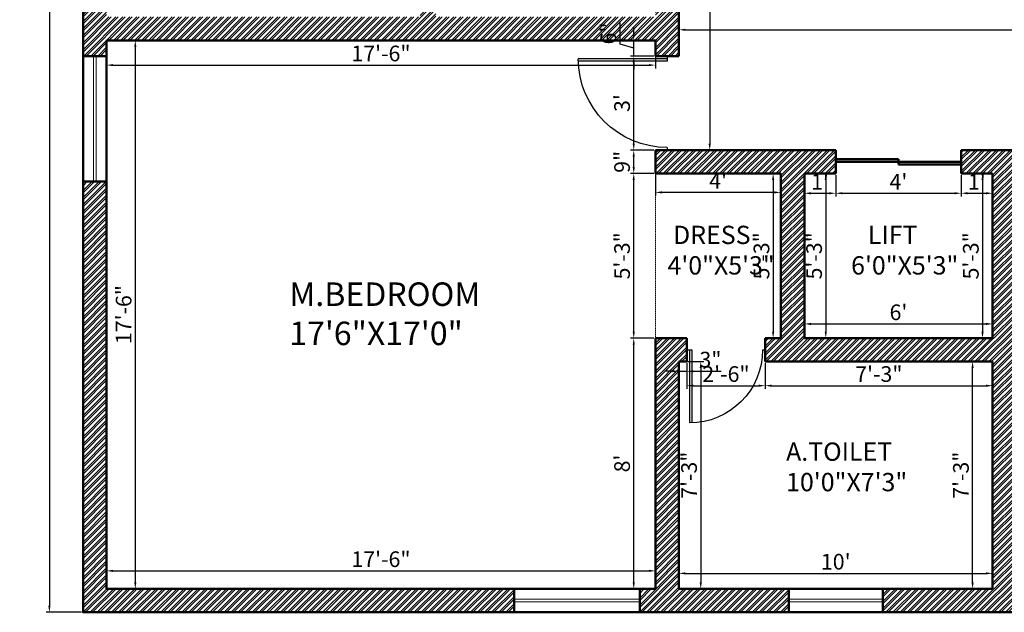
# Model space of a CAD drawing. Units: inches. Extents: x 3590 to 5167, y 65 to 1917.
# Tile 13 of 100: x 3621 to 3998, y 735 to 962. Entities that reach past the tile are written whole.
import ezdxf

# ---------------------------------------------------------------- set-up
doc = ezdxf.new("R2010")
doc.units = ezdxf.units.IN
doc.linetypes.add('DASHED', pattern=[0.75, 0.5, -0.25])
for name, color, linetype, lineweight in [('A-ANNO-DIMS', 2, 'Continuous', 18), ('A-AREA-IDEN', 7, 'Continuous', 18), ('A-DOOR', 3, 'Continuous', 25), ('A-GLAZ', 4, 'Continuous', 18), ('A-WALL', 7, 'Continuous', 50), ('A-WALL-PATT', 251, 'Continuous', 13), ('S-BEAM-OVHD', 7, 'DASHED', 18)]:
    doc.layers.add(name, color=color, linetype=linetype, lineweight=lineweight)
doc.styles.get("Standard").update_dxf_attribs({"font": 'arial.ttf'})
doc.dimstyles.new('ISO-25', dxfattribs={"dimtxt": 9, "dimasz": 2.5, "dimexe": 1.25, "dimexo": 0.625, "dimtad": 1, "dimdec": 1, "dimlunit": 3, "dimtxsty": 'Standard', "dimcen": 2.5, "dimadec": 0, "dimazin": 0, "dimtfac": 1, "dimtdec": 1, "dimtmove": 0, "dimatfit": 3, "dimfxl": 1, "dimarcsym": 0})

# ---------------------------------------------------------------- blocks, each defined once
blk = doc.blocks.new('*D10')
at = {"layer": 'A-ANNO-DIMS', "color": 0, "lineweight": -2, "transparency": 16777216}
for p, q in [((3644.89, 1215.35), (3631.39, 1215.35)), ((3632.64, 1212.85), (3632.64, 737.85)), ((3644.89, 735.35), (3631.39, 735.35))]:
    blk.add_line(p, q, dxfattribs=at)
at = {"layer": 'A-ANNO-DIMS', "color": 0, "transparency": 16777216}
for points in [[(3632.22, 1212.85), (3633.06, 1212.85), (3632.64, 1215.35)], [(3632.22, 737.85), (3633.06, 737.85), (3632.64, 735.35)]]:
    blk.add_solid(points, dxfattribs=at)
at = {"layer": 'Defpoints', "color": 0, "transparency": 16777216}
for p in [(3645.51, 1215.35), (3632.64, 735.35), (3645.51, 735.35)]:
    blk.add_point(p, dxfattribs=at)
at = {"layer": 'A-ANNO-DIMS', "color": 0, "transparency": 16777216, "insert": (3627.42, 975.35), "char_height": 9, "attachment_point": 5, "rotation": 90}
blk.add_mtext("40'", dxfattribs=at)
blk = doc.blocks.new('D2')
for p, q in [((1, 0), (1, 28)), ((2, 0), (2, 27.98)), ((0, 0), (2, 0)), ((29, 0), (30, 0))]:
    blk.add_line(p, q)
at = {"ltscale": 0.5}
blk.add_arc((1, 0), 28, 0, 90, dxfattribs=at)
blk = doc.blocks.new('D1')
for p, q in [((1, 0), (1, 34)), ((2, 0), (2, 33.99)), ((0, 0), (2, 0)), ((35, 0), (36, 0))]:
    blk.add_line(p, q)
at = {"ltscale": 0.5}
blk.add_arc((1, 0), 34, 0, 90, dxfattribs=at)
blk = doc.blocks.new('*D35')
at = {"layer": 'A-ANNO-DIMS', "color": 0, "lineweight": -2, "transparency": 16777216}
for p, q in [((3654.51, 953.72), (3654.51, 943.63)), ((3864.51, 953.72), (3864.51, 943.63)), ((3657.01, 944.88), (3862.01, 944.88))]:
    blk.add_line(p, q, dxfattribs=at)
at = {"layer": 'A-ANNO-DIMS', "color": 0, "transparency": 16777216}
for points in [[(3657.01, 945.3), (3657.01, 944.47), (3654.51, 944.88)], [(3862.01, 945.3), (3862.01, 944.47), (3864.51, 944.88)]]:
    blk.add_solid(points, dxfattribs=at)
at = {"layer": 'Defpoints', "color": 0, "transparency": 16777216}
for p in [(3654.51, 954.35), (3864.51, 954.35), (3864.51, 944.88)]:
    blk.add_point(p, dxfattribs=at)
at = {"layer": 'A-ANNO-DIMS', "color": 0, "transparency": 16777216, "insert": (3759.51, 948.57), "char_height": 6, "attachment_point": 5}
blk.add_mtext('17\'-6"', dxfattribs=at)
blk = doc.blocks.new('*D36')
at = {"layer": 'A-ANNO-DIMS', "color": 0, "lineweight": -2, "transparency": 16777216}
for p, q in [((3655.14, 954.35), (3666.77, 954.35)), ((3665.52, 951.85), (3665.52, 746.85)), ((3655.14, 744.35), (3666.77, 744.35))]:
    blk.add_line(p, q, dxfattribs=at)
at = {"layer": 'A-ANNO-DIMS', "color": 0, "transparency": 16777216}
for points in [[(3665.1, 951.85), (3665.94, 951.85), (3665.52, 954.35)], [(3665.1, 746.85), (3665.94, 746.85), (3665.52, 744.35)]]:
    blk.add_solid(points, dxfattribs=at)
at = {"layer": 'Defpoints', "color": 0, "transparency": 16777216}
for p in [(3654.51, 954.35), (3654.51, 744.35), (3665.52, 744.35)]:
    blk.add_point(p, dxfattribs=at)
at = {"layer": 'A-ANNO-DIMS', "color": 0, "transparency": 16777216, "insert": (3661.83, 849.35), "char_height": 6, "attachment_point": 5, "rotation": 90}
blk.add_mtext('17\'-6"', dxfattribs=at)
blk = doc.blocks.new('*D37')
at = {"layer": 'A-ANNO-DIMS', "color": 0, "lineweight": -2, "transparency": 16777216}
for p, q in [((3654.51, 744.97), (3654.51, 752.47)), ((3657.01, 751.22), (3862.01, 751.22)), ((3864.51, 744.97), (3864.51, 752.47))]:
    blk.add_line(p, q, dxfattribs=at)
at = {"layer": 'A-ANNO-DIMS', "color": 0, "transparency": 16777216}
for points in [[(3657.01, 751.64), (3657.01, 750.81), (3654.51, 751.22)], [(3862.01, 751.64), (3862.01, 750.81), (3864.51, 751.22)]]:
    blk.add_solid(points, dxfattribs=at)
at = {"layer": 'Defpoints', "color": 0, "transparency": 16777216}
for p in [(3864.51, 751.22), (3654.51, 744.35), (3864.51, 744.35)]:
    blk.add_point(p, dxfattribs=at)
at = {"layer": 'A-ANNO-DIMS', "color": 0, "transparency": 16777216, "insert": (3759.51, 754.91), "char_height": 6, "attachment_point": 5}
blk.add_mtext('17\'-6"', dxfattribs=at)
blk = doc.blocks.new('*D38')
at = {"layer": 'A-ANNO-DIMS', "color": 0, "lineweight": -2, "transparency": 16777216}
for p, q in [((3863.89, 840.35), (3854.98, 840.35)), ((3856.23, 746.85), (3856.23, 837.85)), ((3863.89, 744.35), (3854.98, 744.35))]:
    blk.add_line(p, q, dxfattribs=at)
at = {"layer": 'A-ANNO-DIMS', "color": 0, "transparency": 16777216}
for points in [[(3855.81, 837.85), (3856.64, 837.85), (3856.23, 840.35)], [(3855.81, 746.85), (3856.64, 746.85), (3856.23, 744.35)]]:
    blk.add_solid(points, dxfattribs=at)
at = {"layer": 'Defpoints', "color": 0, "transparency": 16777216}
for p in [(3856.23, 840.35), (3864.51, 840.35), (3864.51, 744.35)]:
    blk.add_point(p, dxfattribs=at)
at = {"layer": 'A-ANNO-DIMS', "color": 0, "transparency": 16777216, "insert": (3852.54, 792.35), "char_height": 6, "attachment_point": 5, "rotation": 90}
blk.add_mtext("8'", dxfattribs=at)
blk = doc.blocks.new('*D39')
at = {"layer": 'A-ANNO-DIMS', "color": 0, "lineweight": -2, "transparency": 16777216}
for p, q in [((3863.89, 903.35), (3854.98, 903.35)), ((3856.23, 842.85), (3856.23, 900.85)), ((3863.89, 840.35), (3854.98, 840.35))]:
    blk.add_line(p, q, dxfattribs=at)
at = {"layer": 'A-ANNO-DIMS', "color": 0, "transparency": 16777216}
for points in [[(3855.81, 900.85), (3856.64, 900.85), (3856.23, 903.35)], [(3855.81, 842.85), (3856.64, 842.85), (3856.23, 840.35)]]:
    blk.add_solid(points, dxfattribs=at)
at = {"layer": 'Defpoints', "color": 0, "transparency": 16777216}
for p in [(3856.23, 903.35), (3864.51, 903.35), (3864.51, 840.35)]:
    blk.add_point(p, dxfattribs=at)
at = {"layer": 'A-ANNO-DIMS', "color": 0, "transparency": 16777216, "insert": (3852.54, 871.85), "char_height": 6, "attachment_point": 5, "rotation": 90}
blk.add_mtext('5\'-3"', dxfattribs=at)
blk = doc.blocks.new('*D40')
at = {"layer": 'A-ANNO-DIMS', "color": 0, "lineweight": -2, "transparency": 16777216}
for p, q in [((3863.89, 912.35), (3854.98, 912.35)), ((3856.23, 905.85), (3856.23, 909.85)), ((3863.89, 903.35), (3854.98, 903.35))]:
    blk.add_line(p, q, dxfattribs=at)
at = {"layer": 'A-ANNO-DIMS', "color": 0, "transparency": 16777216}
for points in [[(3855.81, 909.85), (3856.64, 909.85), (3856.23, 912.35)], [(3855.81, 905.85), (3856.64, 905.85), (3856.23, 903.35)]]:
    blk.add_solid(points, dxfattribs=at)
at = {"layer": 'Defpoints', "color": 0, "transparency": 16777216}
for p in [(3856.23, 912.35), (3864.51, 912.35), (3864.51, 903.35)]:
    blk.add_point(p, dxfattribs=at)
at = {"layer": 'A-ANNO-DIMS', "color": 0, "transparency": 16777216, "insert": (3852.54, 907.85), "char_height": 6, "attachment_point": 5, "rotation": 90}
blk.add_mtext('9"', dxfattribs=at)
blk = doc.blocks.new('*D41')
at = {"layer": 'A-ANNO-DIMS', "color": 0, "lineweight": -2, "transparency": 16777216}
for p, q in [((3863.89, 948.35), (3854.98, 948.35)), ((3856.23, 914.85), (3856.23, 945.85)), ((3863.89, 912.35), (3854.98, 912.35))]:
    blk.add_line(p, q, dxfattribs=at)
at = {"layer": 'A-ANNO-DIMS', "color": 0, "transparency": 16777216}
for points in [[(3855.81, 945.85), (3856.64, 945.85), (3856.23, 948.35)], [(3855.81, 914.85), (3856.64, 914.85), (3856.23, 912.35)]]:
    blk.add_solid(points, dxfattribs=at)
at = {"layer": 'Defpoints', "color": 0, "transparency": 16777216}
for p in [(3856.23, 948.35), (3864.51, 948.35), (3864.51, 912.35)]:
    blk.add_point(p, dxfattribs=at)
at = {"layer": 'A-ANNO-DIMS', "color": 0, "transparency": 16777216, "insert": (3852.54, 930.35), "char_height": 6, "attachment_point": 5, "rotation": 90}
blk.add_mtext("3'", dxfattribs=at)
blk = doc.blocks.new('*D42')
at = {"layer": 'A-ANNO-DIMS', "color": 0, "lineweight": -2, "transparency": 16777216}
for p, q in [((3850.98, 952.92), (3850.98, 961.1)), ((3856.23, 956.85), (3856.23, 959.35)), ((3863.89, 954.35), (3854.98, 954.35)), ((3856.23, 948.35), (3856.23, 954.35)), ((3856.23, 948.35), (3856.23, 954.35)), ((3856.23, 951.35), (3850.98, 952.92)), ((3863.89, 948.35), (3854.98, 948.35)), ((3856.23, 945.85), (3856.23, 943.35))]:
    blk.add_line(p, q, dxfattribs=at)
at = {"layer": 'A-ANNO-DIMS', "color": 0, "transparency": 16777216}
for points in [[(3855.81, 956.85), (3856.64, 956.85), (3856.23, 954.35)], [(3855.81, 945.85), (3856.64, 945.85), (3856.23, 948.35)]]:
    blk.add_solid(points, dxfattribs=at)
at = {"layer": 'Defpoints', "color": 0, "transparency": 16777216}
for p in [(3856.23, 954.35), (3864.51, 954.35), (3864.51, 948.35)]:
    blk.add_point(p, dxfattribs=at)
at = {"layer": 'A-ANNO-DIMS', "color": 0, "transparency": 16777216, "insert": (3847.29, 957.01), "char_height": 6, "attachment_point": 5, "rotation": 90}
blk.add_mtext('6"', dxfattribs=at)
blk = doc.blocks.new('*D43')
at = {"layer": 'A-ANNO-DIMS', "color": 0, "lineweight": -2, "transparency": 16777216}
for p, q in [((3864.51, 902.72), (3864.51, 894.9)), ((3912.51, 902.72), (3912.51, 894.9)), ((3910.01, 896.15), (3867.01, 896.15))]:
    blk.add_line(p, q, dxfattribs=at)
at = {"layer": 'A-ANNO-DIMS', "color": 0, "transparency": 16777216}
for points in [[(3867.01, 896.56), (3867.01, 895.73), (3864.51, 896.15)], [(3910.01, 896.56), (3910.01, 895.73), (3912.51, 896.15)]]:
    blk.add_solid(points, dxfattribs=at)
at = {"layer": 'Defpoints', "color": 0, "transparency": 16777216}
for p in [(3864.51, 903.35), (3912.51, 903.35), (3864.51, 896.15)]:
    blk.add_point(p, dxfattribs=at)
at = {"layer": 'A-ANNO-DIMS', "color": 0, "transparency": 16777216, "insert": (3888.51, 899.77), "char_height": 6, "attachment_point": 5}
blk.add_mtext("4'", dxfattribs=at)
blk = doc.blocks.new('*D44')
at = {"layer": 'A-ANNO-DIMS', "color": 0, "lineweight": -2, "transparency": 16777216}
for p, q in [((3911.89, 903.35), (3908.31, 903.35)), ((3909.56, 900.85), (3909.56, 842.85)), ((3911.89, 840.35), (3908.31, 840.35))]:
    blk.add_line(p, q, dxfattribs=at)
at = {"layer": 'A-ANNO-DIMS', "color": 0, "transparency": 16777216}
for points in [[(3909.14, 900.85), (3909.98, 900.85), (3909.56, 903.35)], [(3909.14, 842.85), (3909.98, 842.85), (3909.56, 840.35)]]:
    blk.add_solid(points, dxfattribs=at)
at = {"layer": 'Defpoints', "color": 0, "transparency": 16777216}
for p in [(3912.51, 903.35), (3909.56, 840.35), (3912.51, 840.35)]:
    blk.add_point(p, dxfattribs=at)
at = {"layer": 'A-ANNO-DIMS', "color": 0, "transparency": 16777216, "insert": (3905.87, 871.85), "char_height": 6, "attachment_point": 5, "rotation": 90}
blk.add_mtext('5\'-3"', dxfattribs=at)
blk = doc.blocks.new('*D45')
at = {"layer": 'A-ANNO-DIMS', "color": 0, "lineweight": -2, "transparency": 16777216}
for p, q in [((3873.51, 830.72), (3873.51, 826.4)), ((3876.51, 830.72), (3876.51, 826.4)), ((3871.01, 827.65), (3868.51, 827.65)), ((3873.51, 827.65), (3876.51, 827.65)), ((3879.01, 827.65), (3889.65, 827.65))]:
    blk.add_line(p, q, dxfattribs=at)
at = {"layer": 'A-ANNO-DIMS', "color": 0, "transparency": 16777216}
for points in [[(3871.01, 828.07), (3871.01, 827.24), (3873.51, 827.65)], [(3879.01, 828.07), (3879.01, 827.24), (3876.51, 827.65)]]:
    blk.add_solid(points, dxfattribs=at)
at = {"layer": 'Defpoints', "color": 0, "transparency": 16777216}
for p in [(3873.51, 831.35), (3876.51, 831.35), (3876.51, 827.65)]:
    blk.add_point(p, dxfattribs=at)
at = {"layer": 'A-ANNO-DIMS', "color": 0, "transparency": 16777216, "insert": (3885.58, 831.34), "char_height": 6, "attachment_point": 5}
blk.add_mtext('3"', dxfattribs=at)
blk = doc.blocks.new('*D46')
at = {"layer": 'A-ANNO-DIMS', "color": 0, "lineweight": -2, "transparency": 16777216}
for p, q in [((3876.51, 830.72), (3876.51, 820.87)), ((3906.51, 830.72), (3906.51, 820.87)), ((3879.01, 822.12), (3904.01, 822.12))]:
    blk.add_line(p, q, dxfattribs=at)
at = {"layer": 'A-ANNO-DIMS', "color": 0, "transparency": 16777216}
for points in [[(3879.01, 822.54), (3879.01, 821.7), (3876.51, 822.12)], [(3904.01, 822.54), (3904.01, 821.7), (3906.51, 822.12)]]:
    blk.add_solid(points, dxfattribs=at)
at = {"layer": 'Defpoints', "color": 0, "transparency": 16777216}
for p in [(3876.51, 831.35), (3906.51, 831.35), (3906.51, 822.12)]:
    blk.add_point(p, dxfattribs=at)
at = {"layer": 'A-ANNO-DIMS', "color": 0, "transparency": 16777216, "insert": (3891.51, 825.81), "char_height": 6, "attachment_point": 5}
blk.add_mtext('2\'-6"', dxfattribs=at)
blk = doc.blocks.new('*D47')
at = {"layer": 'A-ANNO-DIMS', "color": 0, "lineweight": -2, "transparency": 16777216}
for p, q in [((3906.51, 830.72), (3906.51, 820.87)), ((3993.51, 830.72), (3993.51, 820.87)), ((3909.01, 822.12), (3991.01, 822.12))]:
    blk.add_line(p, q, dxfattribs=at)
at = {"layer": 'A-ANNO-DIMS', "color": 0, "transparency": 16777216}
for points in [[(3909.01, 822.54), (3909.01, 821.7), (3906.51, 822.12)], [(3991.01, 822.54), (3991.01, 821.7), (3993.51, 822.12)]]:
    blk.add_solid(points, dxfattribs=at)
at = {"layer": 'Defpoints', "color": 0, "transparency": 16777216}
for p in [(3906.51, 831.35), (3993.51, 831.35), (3993.51, 822.12)]:
    blk.add_point(p, dxfattribs=at)
at = {"layer": 'A-ANNO-DIMS', "color": 0, "transparency": 16777216, "insert": (3950.01, 825.81), "char_height": 6, "attachment_point": 5}
blk.add_mtext('7\'-3"', dxfattribs=at)
blk = doc.blocks.new('*D48')
at = {"layer": 'A-ANNO-DIMS', "color": 0, "lineweight": -2, "transparency": 16777216}
for p, q in [((3874.14, 831.35), (3883.11, 831.35)), ((3881.86, 828.85), (3881.86, 746.85)), ((3874.14, 744.35), (3883.11, 744.35))]:
    blk.add_line(p, q, dxfattribs=at)
at = {"layer": 'A-ANNO-DIMS', "color": 0, "transparency": 16777216}
for points in [[(3881.44, 828.85), (3882.28, 828.85), (3881.86, 831.35)], [(3881.44, 746.85), (3882.28, 746.85), (3881.86, 744.35)]]:
    blk.add_solid(points, dxfattribs=at)
at = {"layer": 'Defpoints', "color": 0, "transparency": 16777216}
for p in [(3873.51, 831.35), (3873.51, 744.35), (3881.86, 744.35)]:
    blk.add_point(p, dxfattribs=at)
at = {"layer": 'A-ANNO-DIMS', "color": 0, "transparency": 16777216, "insert": (3878.17, 787.85), "char_height": 6, "attachment_point": 5, "rotation": 90}
blk.add_mtext('7\'-3"', dxfattribs=at)
blk = doc.blocks.new('*D49')
at = {"layer": 'A-ANNO-DIMS', "color": 0, "lineweight": -2, "transparency": 16777216}
for p, q in [((3873.51, 744.97), (3873.51, 751.51)), ((3876.01, 750.26), (3991.01, 750.26)), ((3993.51, 744.97), (3993.51, 751.51))]:
    blk.add_line(p, q, dxfattribs=at)
at = {"layer": 'A-ANNO-DIMS', "color": 0, "transparency": 16777216}
for points in [[(3876.01, 750.68), (3876.01, 749.84), (3873.51, 750.26)], [(3991.01, 750.68), (3991.01, 749.84), (3993.51, 750.26)]]:
    blk.add_solid(points, dxfattribs=at)
at = {"layer": 'Defpoints', "color": 0, "transparency": 16777216}
for p in [(3993.51, 750.26), (3873.51, 744.35), (3993.51, 744.35)]:
    blk.add_point(p, dxfattribs=at)
at = {"layer": 'A-ANNO-DIMS', "color": 0, "transparency": 16777216, "insert": (3933.51, 753.95), "char_height": 6, "attachment_point": 5}
blk.add_mtext("10'", dxfattribs=at)
blk = doc.blocks.new('*D50')
at = {"layer": 'A-ANNO-DIMS', "color": 0, "lineweight": -2, "transparency": 16777216}
for p, q in [((3992.89, 831.35), (3984.62, 831.35)), ((3985.87, 746.85), (3985.87, 828.85)), ((3992.89, 744.35), (3984.62, 744.35))]:
    blk.add_line(p, q, dxfattribs=at)
at = {"layer": 'A-ANNO-DIMS', "color": 0, "transparency": 16777216}
for points in [[(3985.45, 828.85), (3986.29, 828.85), (3985.87, 831.35)], [(3985.45, 746.85), (3986.29, 746.85), (3985.87, 744.35)]]:
    blk.add_solid(points, dxfattribs=at)
at = {"layer": 'Defpoints', "color": 0, "transparency": 16777216}
for p in [(3985.87, 831.35), (3993.51, 831.35), (3993.51, 744.35)]:
    blk.add_point(p, dxfattribs=at)
at = {"layer": 'A-ANNO-DIMS', "color": 0, "transparency": 16777216, "insert": (3982.18, 787.85), "char_height": 6, "attachment_point": 5, "rotation": 90}
blk.add_mtext('7\'-3"', dxfattribs=at)
blk = doc.blocks.new('*D51')
at = {"layer": 'A-ANNO-DIMS', "color": 0, "lineweight": -2, "transparency": 16777216}
for p, q in [((3921.51, 840.97), (3921.51, 847.03)), ((3924.01, 845.78), (3991.01, 845.78)), ((3993.51, 840.97), (3993.51, 847.03))]:
    blk.add_line(p, q, dxfattribs=at)
at = {"layer": 'A-ANNO-DIMS', "color": 0, "transparency": 16777216}
for points in [[(3924.01, 846.2), (3924.01, 845.37), (3921.51, 845.78)], [(3991.01, 846.2), (3991.01, 845.37), (3993.51, 845.78)]]:
    blk.add_solid(points, dxfattribs=at)
at = {"layer": 'Defpoints', "color": 0, "transparency": 16777216}
for p in [(3993.51, 845.78), (3921.51, 840.35), (3993.51, 840.35)]:
    blk.add_point(p, dxfattribs=at)
at = {"layer": 'A-ANNO-DIMS', "color": 0, "transparency": 16777216, "insert": (3957.51, 849.47), "char_height": 6, "attachment_point": 5}
blk.add_mtext("6'", dxfattribs=at)
blk = doc.blocks.new('*D52')
at = {"layer": 'A-ANNO-DIMS', "color": 0, "lineweight": -2, "transparency": 16777216}
for p, q in [((3922.14, 903.35), (3930.95, 903.35)), ((3929.7, 900.85), (3929.7, 842.85)), ((3922.14, 840.35), (3930.95, 840.35))]:
    blk.add_line(p, q, dxfattribs=at)
at = {"layer": 'A-ANNO-DIMS', "color": 0, "transparency": 16777216}
for points in [[(3929.29, 900.85), (3930.12, 900.85), (3929.7, 903.35)], [(3929.29, 842.85), (3930.12, 842.85), (3929.7, 840.35)]]:
    blk.add_solid(points, dxfattribs=at)
at = {"layer": 'Defpoints', "color": 0, "transparency": 16777216}
for p in [(3921.51, 903.35), (3921.51, 840.35), (3929.7, 840.35)]:
    blk.add_point(p, dxfattribs=at)
at = {"layer": 'A-ANNO-DIMS', "color": 0, "transparency": 16777216, "insert": (3926.01, 871.85), "char_height": 6, "attachment_point": 5, "rotation": 90}
blk.add_mtext('5\'-3"', dxfattribs=at)
blk = doc.blocks.new('*D53')
at = {"layer": 'A-ANNO-DIMS', "color": 0, "lineweight": -2, "transparency": 16777216}
for p, q in [((3992.89, 903.35), (3988.42, 903.35)), ((3989.67, 900.85), (3989.67, 842.85)), ((3992.89, 840.35), (3988.42, 840.35))]:
    blk.add_line(p, q, dxfattribs=at)
at = {"layer": 'A-ANNO-DIMS', "color": 0, "transparency": 16777216}
for points in [[(3989.25, 900.85), (3990.09, 900.85), (3989.67, 903.35)], [(3989.25, 842.85), (3990.09, 842.85), (3989.67, 840.35)]]:
    blk.add_solid(points, dxfattribs=at)
at = {"layer": 'Defpoints', "color": 0, "transparency": 16777216}
for p in [(3993.51, 903.35), (3989.67, 840.35), (3993.51, 840.35)]:
    blk.add_point(p, dxfattribs=at)
at = {"layer": 'A-ANNO-DIMS', "color": 0, "transparency": 16777216, "insert": (3985.98, 871.85), "char_height": 6, "attachment_point": 5, "rotation": 90}
blk.add_mtext('5\'-3"', dxfattribs=at)
blk = doc.blocks.new('*D54')
at = {"layer": 'A-ANNO-DIMS', "color": 0, "lineweight": -2, "transparency": 16777216}
for p, q in [((3921.51, 902.72), (3921.51, 894.56)), ((3933.51, 902.72), (3933.51, 894.56)), ((3924.01, 895.81), (3931.01, 895.81))]:
    blk.add_line(p, q, dxfattribs=at)
at = {"layer": 'A-ANNO-DIMS', "color": 0, "transparency": 16777216}
for points in [[(3924.01, 896.23), (3924.01, 895.4), (3921.51, 895.81)], [(3931.01, 896.23), (3931.01, 895.4), (3933.51, 895.81)]]:
    blk.add_solid(points, dxfattribs=at)
at = {"layer": 'Defpoints', "color": 0, "transparency": 16777216}
for p in [(3921.51, 903.35), (3933.51, 903.35), (3933.51, 895.81)]:
    blk.add_point(p, dxfattribs=at)
at = {"layer": 'A-ANNO-DIMS', "color": 0, "transparency": 16777216, "insert": (3927.51, 899.45), "char_height": 6, "attachment_point": 5}
blk.add_mtext("1'", dxfattribs=at)
blk = doc.blocks.new('*D55')
at = {"layer": 'A-ANNO-DIMS', "color": 0, "lineweight": -2, "transparency": 16777216}
for p, q in [((3933.51, 902.72), (3933.51, 894.56)), ((3981.51, 902.72), (3981.51, 894.56)), ((3936.01, 895.81), (3979.01, 895.81))]:
    blk.add_line(p, q, dxfattribs=at)
at = {"layer": 'A-ANNO-DIMS', "color": 0, "transparency": 16777216}
for points in [[(3936.01, 896.23), (3936.01, 895.4), (3933.51, 895.81)], [(3979.01, 896.23), (3979.01, 895.4), (3981.51, 895.81)]]:
    blk.add_solid(points, dxfattribs=at)
at = {"layer": 'Defpoints', "color": 0, "transparency": 16777216}
for p in [(3933.51, 903.35), (3981.51, 903.35), (3981.51, 895.81)]:
    blk.add_point(p, dxfattribs=at)
at = {"layer": 'A-ANNO-DIMS', "color": 0, "transparency": 16777216, "insert": (3957.51, 899.44), "char_height": 6, "attachment_point": 5}
blk.add_mtext("4'", dxfattribs=at)
blk = doc.blocks.new('*D56')
at = {"layer": 'A-ANNO-DIMS', "color": 0, "lineweight": -2, "transparency": 16777216}
for p, q in [((3981.51, 902.72), (3981.51, 894.56)), ((3993.51, 902.72), (3993.51, 894.56)), ((3984.01, 895.81), (3991.01, 895.81))]:
    blk.add_line(p, q, dxfattribs=at)
at = {"layer": 'A-ANNO-DIMS', "color": 0, "transparency": 16777216}
for points in [[(3984.01, 896.23), (3984.01, 895.4), (3981.51, 895.81)], [(3991.01, 896.23), (3991.01, 895.4), (3993.51, 895.81)]]:
    blk.add_solid(points, dxfattribs=at)
at = {"layer": 'Defpoints', "color": 0, "transparency": 16777216}
for p in [(3981.51, 903.35), (3993.51, 903.35), (3993.51, 895.81)]:
    blk.add_point(p, dxfattribs=at)
at = {"layer": 'A-ANNO-DIMS', "color": 0, "transparency": 16777216, "insert": (3987.51, 899.45), "char_height": 6, "attachment_point": 5}
blk.add_mtext("1'", dxfattribs=at)
blk = doc.blocks.new('*D73')
at = {"layer": 'A-ANNO-DIMS', "color": 0, "lineweight": -2, "transparency": 16777216}
for p, q in [((3874.14, 1206.35), (3886.54, 1206.35)), ((3885.29, 1203.85), (3885.29, 914.85)), ((3874.14, 912.35), (3886.54, 912.35))]:
    blk.add_line(p, q, dxfattribs=at)
at = {"layer": 'A-ANNO-DIMS', "color": 0, "transparency": 16777216}
for points in [[(3884.87, 1203.85), (3885.7, 1203.85), (3885.29, 1206.35)], [(3884.87, 914.85), (3885.7, 914.85), (3885.29, 912.35)]]:
    blk.add_solid(points, dxfattribs=at)
at = {"layer": 'Defpoints', "color": 0, "transparency": 16777216}
for p in [(3873.51, 1206.35), (3873.51, 912.35), (3885.29, 912.35)]:
    blk.add_point(p, dxfattribs=at)
at = {"layer": 'A-ANNO-DIMS', "color": 0, "transparency": 16777216, "insert": (3881.6, 1059.35), "char_height": 6, "attachment_point": 5, "rotation": 90}
blk.add_mtext('24\'-6"', dxfattribs=at)
blk = doc.blocks.new('*D74')
at = {"layer": 'A-ANNO-DIMS', "color": 0, "lineweight": -2, "transparency": 16777216}
for p, q in [((3873.51, 948.97), (3873.51, 959.67)), ((3876.01, 958.42), (4147.01, 958.42)), ((4149.51, 945.97), (4149.51, 959.67))]:
    blk.add_line(p, q, dxfattribs=at)
at = {"layer": 'A-ANNO-DIMS', "color": 0, "transparency": 16777216}
for points in [[(3876.01, 958.83), (3876.01, 958), (3873.51, 958.42)], [(4147.01, 958.83), (4147.01, 958), (4149.51, 958.42)]]:
    blk.add_solid(points, dxfattribs=at)
at = {"layer": 'Defpoints', "color": 0, "transparency": 16777216}
for p in [(4149.51, 958.42), (3873.51, 948.35), (4149.51, 945.35)]:
    blk.add_point(p, dxfattribs=at)
at = {"layer": 'A-ANNO-DIMS', "color": 0, "transparency": 16777216, "insert": (4011.51, 962.11), "char_height": 6, "attachment_point": 5}
blk.add_mtext("23'", dxfattribs=at)

msp = doc.modelspace()

# ---------------------------------------------------------------- hatches: boundary and pattern name
at = {"layer": 'A-WALL-PATT', "transparency": 33554687}
h = msp.add_hatch(dxfattribs=at)
h.set_pattern_fill('ANSI32', color=256, scale=0.2)
h.set_pattern_definition([(45, (0, -590.6538), (-1.3470384, 1.3470384), []), (45, (0.898, -590.6538), (-1.3470384, 1.3470384), [])])
h.paths.add_polyline_path([(3768.51, 1215.35), (3645.51, 1215.35), (3645.51, 1194.35), (3654.51, 1194.35), (3654.51, 1206.35), (3671.16, 1206.35), (3768.51, 1206.35)])
h.paths.add_polyline_path([(3909.51, 1215.35), (3816.51, 1215.35), (3816.51, 1206.35), (3864.51, 1206.35), (3864.51, 1200.35), (3873.51, 1200.35), (3873.51, 1206.35), (3909.51, 1206.35)])
h.paths.add_polyline_path([(4053.51, 1215.35), (3969.51, 1215.35), (3969.51, 1206.35), (4053.51, 1206.35)])
h.paths.add_polyline_path([(4215.51, 1215.35), (4113.51, 1215.35), (4113.51, 1206.35), (4206.51, 1206.35), (4206.51, 1200.35), (4215.51, 1200.35)])
h.paths.add_polyline_path([(3654.51, 1146.35), (3645.51, 1146.35), (3645.51, 1029.35), (3654.51, 1029.35), (3654.51, 1059.35), (3741.51, 1059.35), (3741.51, 1065.35), (3654.51, 1065.35)], flags=17)
h.paths.add_polyline_path([(3873.51, 1164.35), (3864.51, 1164.35), (3864.51, 1065.35), (3771.51, 1065.35), (3771.51, 1059.35), (3774.51, 1059.35), (3774.51, 963.35), (3654.51, 963.35), (3654.51, 993.35), (3645.51, 993.35), (3645.51, 948.35), (3654.51, 948.35), (3654.51, 954.35), (3864.51, 954.35), (3864.51, 948.35), (3873.51, 948.35), (3873.51, 993.35), (3864.51, 993.35), (3864.51, 963.35), (3780.51, 963.35), (3780.51, 1059.35), (3864.51, 1059.35), (3864.51, 1029.35), (3873.51, 1029.35)])
h.paths.add_polyline_path([(3654.51, 900.35), (3645.51, 900.35), (3645.51, 735.35), (3810.51, 735.35), (3810.51, 744.35), (3809.96, 744.35), (3654.51, 744.35)])
h.paths.add_polyline_path([(3915.51, 744.35), (3873.51, 744.35), (3873.51, 762.21), (3873.51, 831.35), (3876.51, 831.35), (3876.51, 840.35), (3864.51, 840.35), (3864.51, 744.35), (3858.51, 744.35), (3858.51, 735.35), (3915.51, 735.35)])
h.paths.add_polyline_path([(4028.01, 744.35), (4002.51, 744.35), (4002.51, 912.35), (3981.51, 912.35), (3981.51, 903.35), (3993.51, 903.35), (3993.51, 840.35), (3921.51, 840.35), (3921.51, 903.35), (3933.51, 903.35), (3933.51, 912.35), (3864.51, 912.35), (3864.51, 903.35), (3912.51, 903.35), (3912.51, 840.35), (3906.51, 840.35), (3906.51, 831.35), (3993.51, 831.35), (3993.51, 744.35), (3951.51, 744.35), (3951.51, 735.35), (4028.01, 735.35)])
h.paths.add_polyline_path([(4203.51, 744.35), (4158.51, 744.35), (4158.51, 936.35), (4194.51, 936.35), (4194.51, 945.35), (4149.51, 945.35), (4149.51, 744.35), (4124.01, 744.35), (4124.01, 735.35), (4203.51, 735.35)])
h.paths.add_polyline_path([(4305.51, 975.35), (4296.51, 975.35), (4296.51, 945.35), (4278.64, 945.35), (4260.51, 945.35), (4260.51, 936.35), (4296.51, 936.35), (4296.51, 930.35), (4305.51, 930.35)])
h.paths.add_polyline_path([(4305.51, 882.35), (4296.51, 882.35), (4296.51, 744.35), (4251.51, 744.35), (4251.51, 735.35), (4305.51, 735.35)])
h.paths.add_polyline_path([(4305.51, 1086.35), (4215.51, 1086.35), (4215.51, 1152.35), (4206.51, 1152.35), (4206.51, 1086.35), (4149.51, 1086.35), (4149.51, 1077.35), (4296.51, 1077.35), (4296.51, 1047.35), (4305.51, 1047.35)])

# ---------------------------------------------------------------- linework, layer by layer
at = {"layer": 'A-GLAZ'}
for p, q in [((3649.51, 900.35), (3649.51, 948.35)), ((3650.51, 900.35), (3650.51, 948.35)), ((3858.51, 740.35), (3810.51, 740.35)), ((3858.51, 739.35), (3810.51, 739.35)), ((3951.51, 740.35), (3915.51, 740.35)), ((3951.51, 739.35), (3915.51, 739.35))]:
    msp.add_line(p, q, dxfattribs=at)
at = {"layer": 'A-WALL'}
for p, q in [((3873.51, 948.35), (3873.51, 993.35)), ((3864.51, 954.35), (3654.51, 954.35)), ((3654.51, 744.35), (3654.51, 954.35)), ((3864.51, 948.35), (3864.51, 954.35)), ((3654.51, 948.35), (3645.51, 948.35)), ((3873.51, 948.35), (3864.51, 948.35)), ((3933.51, 912.35), (3864.51, 912.35)), ((3864.51, 903.35), (3864.51, 912.35)), ((3933.51, 903.35), (3933.51, 912.35)), ((4002.51, 912.35), (3981.51, 912.35)), ((3981.51, 903.35), (3981.51, 912.35)), ((3933.51, 908.85), (3957.51, 908.85)), ((3957.51, 908.85), (3957.51, 906.85)), ((3933.51, 907.85), (3981.51, 907.85)), ((3957.51, 906.85), (3981.51, 906.85)), ((3912.51, 903.35), (3864.51, 903.35)), ((3912.51, 840.35), (3912.51, 903.35)), ((3933.51, 903.35), (3921.51, 903.35)), ((3921.51, 840.35), (3921.51, 903.35)), ((3993.51, 903.35), (3981.51, 903.35)), ((3993.51, 840.35), (3993.51, 903.35)), ((3654.51, 900.35), (3645.51, 900.35)), ((3876.51, 840.35), (3864.51, 840.35)), ((3864.51, 744.35), (3864.51, 840.35)), ((3876.51, 831.35), (3876.51, 840.35)), ((3912.51, 840.35), (3906.51, 840.35)), ((3906.51, 831.35), (3906.51, 840.35)), ((3993.51, 840.35), (3921.51, 840.35)), ((3876.51, 831.35), (3873.51, 831.35)), ((3873.51, 744.35), (3873.51, 831.35)), ((3993.51, 831.35), (3906.51, 831.35)), ((3993.51, 744.35), (3993.51, 831.35)), ((3864.51, 744.35), (3654.51, 744.35)), ((3810.51, 735.35), (3810.51, 744.35)), ((3858.51, 735.35), (3858.51, 744.35)), ((3993.51, 744.35), (3873.51, 744.35)), ((3915.51, 744.35), (3915.51, 735.35)), ((3951.51, 744.35), (3951.51, 735.35))]:
    msp.add_line(p, q, dxfattribs=at)
msp.add_lwpolyline([(4305.51, 1086.35), (4305.51, 735.35), (3645.51, 735.35), (3645.51, 1215.35), (4215.51, 1215.35)], dxfattribs=at)
at = {"layer": 'S-BEAM-OVHD'}
msp.add_line((3864.51, 903.35), (3864.51, 840.35), dxfattribs=at)

# ---------------------------------------------------------------- block references
at = {"layer": 'A-DOOR', "xscale": -1}
for name, p, rotation in [('D1', (3869.01, 948.35), 90), ('D2', (3876.51, 835.85), 180)]:
    msp.add_blockref(name, p, dxfattribs=dict(at, rotation=rotation))

# ---------------------------------------------------------------- texts
at = {"layer": 'A-AREA-IDEN', "attachment_point": 1}
for s, insert, char_height in [('{\\fTimes New Roman|b0|i0|c0|p18; DRESS\\P4\'0"X5\'3"}', (3869.13, 883.37), 7), ('{\\fTimes New Roman|b0|i0|c0|p18;   LIFT\\P6\'0"X5\'3"}', (3939.39, 883.37), 7), ('{\\fTimes New Roman|b0|i0|c0|p18;M.BEDROOM\\P 17\'6"X17\'0"}', (3724.44, 861.67), 9), ('{\\fTimes New Roman|b0|i0|c0|p18;A.TOILET\\P10\'0"X7\'3"}', (3914.52, 800.38), 7)]:
    msp.add_mtext_dynamic_manual_height_columns(s, width=67.3508, gutter_width=12.5, heights=[0], dxfattribs=dict(at, insert=insert, char_height=char_height))

# ---------------------------------------------------------------- dimensions: what is measured, and where the dimension line sits
at = {"layer": 'A-ANNO-DIMS'}
for base, p1, p2, override, picture, middle in [((3632.64, 735.35), (3645.51, 1215.35), (3645.51, 735.35), {"dimclrd": 0, "dimclre": 0, "dimclrt": 0}, '*D10', (3627.42, 975.35)), ((3885.29, 912.35), (3873.51, 1206.35), (3873.51, 912.35), {"dimtxt": 6, "dimclrd": 0, "dimclre": 0, "dimclrt": 0}, '*D73', (3881.6, 1059.35)), ((3856.23, 954.35), (3864.51, 948.35), (3864.51, 954.35), {"dimtxt": 6, "dimclrd": 0, "dimclre": 0, "dimclrt": 0, "dimtmove": 1}, '*D42', (3847.29, 953.55)), ((3665.52, 744.35), (3654.51, 954.35), (3654.51, 744.35), {"dimtxt": 6, "dimclrd": 0, "dimclre": 0, "dimclrt": 0}, '*D36', (3661.83, 849.35)), ((3856.23, 948.35), (3864.51, 912.35), (3864.51, 948.35), {"dimtxt": 6, "dimclrd": 0, "dimclre": 0, "dimclrt": 0, "dimtmove": 1}, '*D41', (3852.54, 930.35)), ((3856.23, 912.35), (3864.51, 903.35), (3864.51, 912.35), {"dimtxt": 6, "dimclrd": 0, "dimclre": 0, "dimclrt": 0, "dimtmove": 1}, '*D40', (3852.54, 907.85)), ((3856.23, 903.35), (3864.51, 840.35), (3864.51, 903.35), {"dimtxt": 6, "dimclrd": 0, "dimclre": 0, "dimclrt": 0, "dimtmove": 1}, '*D39', (3852.54, 871.85)), ((3909.56, 840.35), (3912.51, 903.35), (3912.51, 840.35), {"dimtxt": 6, "dimclrd": 0, "dimclre": 0, "dimclrt": 0}, '*D44', (3905.87, 871.85)), ((3929.7, 840.35), (3921.51, 903.35), (3921.51, 840.35), {"dimtxt": 6, "dimclrd": 0, "dimclre": 0, "dimclrt": 0}, '*D52', (3926.01, 871.85)), ((3989.67, 840.35), (3993.51, 903.35), (3993.51, 840.35), {"dimtxt": 6, "dimclrd": 0, "dimclre": 0, "dimclrt": 0}, '*D53', (3985.98, 871.85)), ((3856.23, 840.35), (3864.51, 744.35), (3864.51, 840.35), {"dimtxt": 6, "dimclrd": 0, "dimclre": 0, "dimclrt": 0}, '*D38', (3852.54, 792.35)), ((3881.86, 744.35), (3873.51, 831.35), (3873.51, 744.35), {"dimtxt": 6, "dimclrd": 0, "dimclre": 0, "dimclrt": 0}, '*D48', (3878.17, 787.85)), ((3985.87, 831.35), (3993.51, 744.35), (3993.51, 831.35), {"dimtxt": 6, "dimclrd": 0, "dimclre": 0, "dimclrt": 0}, '*D50', (3982.18, 787.85))]:
    dim = msp.add_linear_dim(base=base, p1=p1, p2=p2, angle=90, dimstyle='ISO-25', override=override, dxfattribs=at)
    dim.commit()
    dim.dimension.update_dxf_attribs({"geometry": picture, "text_midpoint": middle})
for base, p1, p2, override, picture, middle in [((4149.51, 958.42), (3873.51, 948.35), (4149.51, 945.35), {"dimtxt": 6, "dimclrd": 0, "dimclre": 0, "dimclrt": 0}, '*D74', (4011.51, 962.11)), ((3864.51, 944.88), (3654.51, 954.35), (3864.51, 954.35), {"dimtxt": 6, "dimclrd": 0, "dimclre": 0, "dimclrt": 0}, '*D35', (3759.51, 948.57)), ((3864.51, 896.15), (3912.51, 903.35), (3864.51, 903.35), {"dimtxt": 6, "dimclrd": 0, "dimclre": 0, "dimclrt": 0}, '*D43', (3888.51, 899.77)), ((3933.51, 895.81), (3921.51, 903.35), (3933.51, 903.35), {"dimtxt": 6, "dimclrd": 0, "dimclre": 0, "dimclrt": 0}, '*D54', (3927.51, 899.45)), ((3981.51, 895.81), (3933.51, 903.35), (3981.51, 903.35), {"dimtxt": 6, "dimclrd": 0, "dimclre": 0, "dimclrt": 0, "dimtmove": 1}, '*D55', (3957.51, 899.44)), ((3993.51, 895.81), (3981.51, 903.35), (3993.51, 903.35), {"dimtxt": 6, "dimclrd": 0, "dimclre": 0, "dimclrt": 0, "dimtmove": 1}, '*D56', (3987.51, 899.45)), ((3993.51, 845.78), (3921.51, 840.35), (3993.51, 840.35), {"dimtxt": 6, "dimclrd": 0, "dimclre": 0, "dimclrt": 0}, '*D51', (3957.51, 849.47)), ((3876.51, 827.65), (3873.51, 831.35), (3876.51, 831.35), {"dimtxt": 6, "dimclrd": 0, "dimclre": 0, "dimclrt": 0}, '*D45', (3885.58, 831.34)), ((3906.51, 822.12), (3876.51, 831.35), (3906.51, 831.35), {"dimtxt": 6, "dimclrd": 0, "dimclre": 0, "dimclrt": 0, "dimtmove": 1}, '*D46', (3891.51, 825.81)), ((3993.51, 822.12), (3906.51, 831.35), (3993.51, 831.35), {"dimtxt": 6, "dimclrd": 0, "dimclre": 0, "dimclrt": 0, "dimtmove": 1}, '*D47', (3950.01, 825.81)), ((3864.51, 751.22), (3654.51, 744.35), (3864.51, 744.35), {"dimtxt": 6, "dimclrd": 0, "dimclre": 0, "dimclrt": 0}, '*D37', (3759.51, 754.91)), ((3993.51, 750.26), (3873.51, 744.35), (3993.51, 744.35), {"dimtxt": 6, "dimclrd": 0, "dimclre": 0, "dimclrt": 0}, '*D49', (3933.51, 753.95))]:
    dim = msp.add_linear_dim(base=base, p1=p1, p2=p2, dimstyle='ISO-25', override=override, dxfattribs=at)
    dim.commit()
    dim.dimension.update_dxf_attribs({"geometry": picture, "text_midpoint": middle})

doc.saveas('drawing.dxf')
